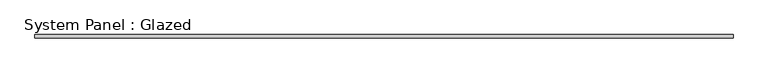
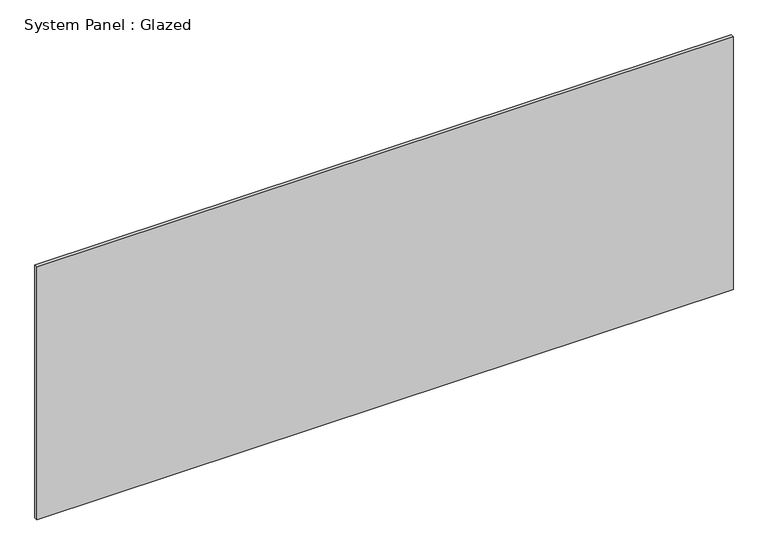
"""IFC4 building model written with IfcOpenShell, lengths in millimetres: plate geometry, System Panel : Glazed."""

from ifc_helpers import new_model, si_unit, origin, origin_with_axes, place, context, project, spatial, polyline, outline, extrude, source, transform, mapped, element, save


def system_panel_glazed_95ff72d9(model_context):
    return source(origin(), model_context, "Body", "SweptSolid", [
        extrude(outline(polyline([(2591.5717045, 19.05), (-2591.5717045, 19.05), (-2591.5717045, 44.45), (2591.5717045, 44.45), (2591.5717045, 19.05)])), origin_with_axes(), (0.0, 0.0, 1.0), 1990.8954044),
    ])


if __name__ == "__main__":
    model = new_model("IFC4")
    model_context = context("Model", 3, world=origin())
    ifc_project = project(units=[si_unit("LENGTHUNIT", "METRE", prefix="MILLI")], contexts=[model_context])
    site = spatial("IfcSite", under=ifc_project)
    building = spatial("IfcBuilding", under=site)
    placement = place(None, origin())
    system_panel_glazed_shape = system_panel_glazed_95ff72d9(model_context)
    element("IfcPlate", 1, ObjectType="System Panel : Glazed", at=placement, inside=building, context=model_context, shape_type="MappedRepresentation", body=[
        mapped(system_panel_glazed_shape, transform((0.0, 0.0, 0.0), x_axis=(1.0, 0.0, 0.0), y_axis=(0.0, 1.0, 0.0), z_axis=(0.0, 0.0, 1.0))),
    ])
    save(model, "model.ifc")

# Revit data of these elements
# Type "System Panel : Glazed"
#   Construction Type Id = "GSP4R"
#   Analytic Construction = "1/8 in Pilkington single glazing"
#   Visual Light Transmittance = 0.9
#   Solar Heat Gain Coefficient = 0.86
#   Heat Transfer Coefficient (U) = 1.18115 BTU/(h·ft²·°F)
#   Define Thermal Properties by = 1
# Element 1 (IfcPlate, "System Panel : Glazed")
#   Materials on its faces: "Glass"
# Materials
#   "Glass": class "Glass", colour RGB 0 128 192, transparency 0.75, Description = "Soda Lime Glass", Cost = 0
